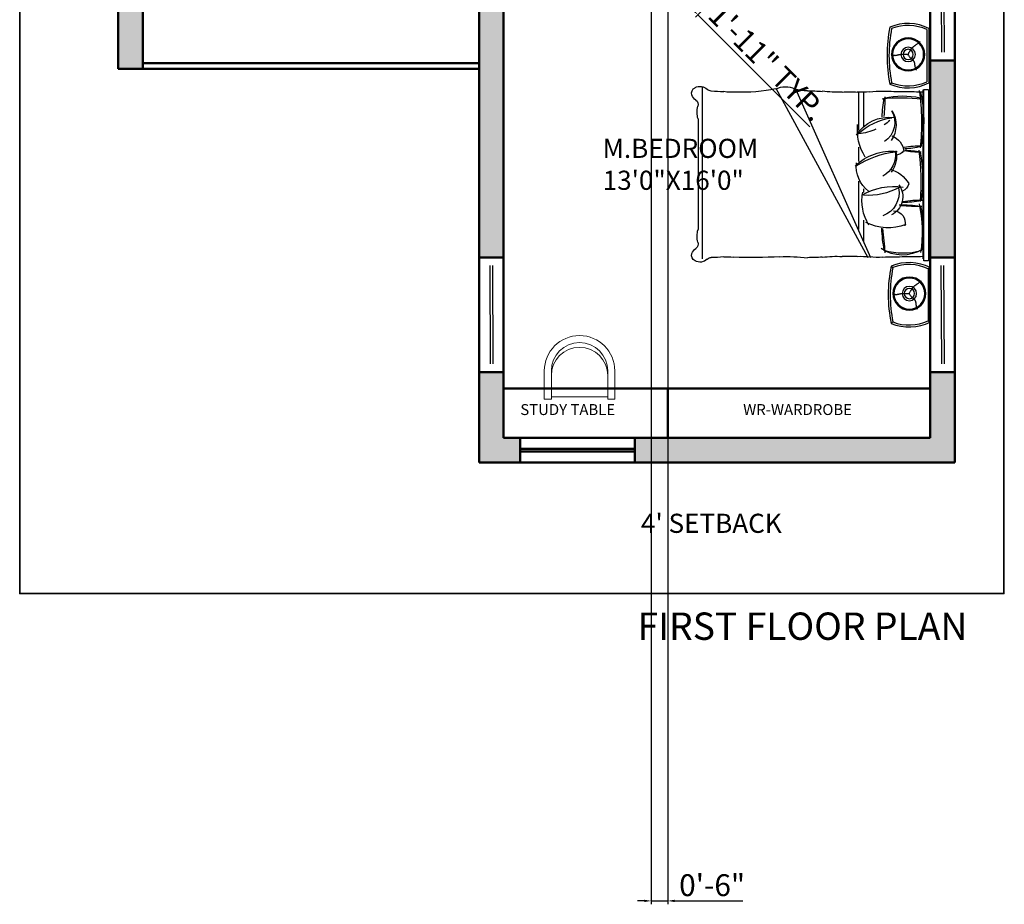
# Model space of a CAD drawing. Units: inches. Extents: x 1986 to 21484, y -1816 to 2016.
# Tile 4 of 85: x 2500 to 2860, y 953 to 1277. Entities that reach past the tile are written whole.
import ezdxf

# ---------------------------------------------------------------- set-up
doc = ezdxf.new("R2010")
doc.units = ezdxf.units.IN
for name, color, linetype, lineweight in [('A-ANNO-DIMS', 2, 'Continuous', 18), ('A-ANNO-TEXT', 7, 'Continuous', 18), ('A-AREA-IDEN', 3, 'Continuous', 18), ('A-FLOR-FIXT', 8, 'Continuous', 18), ('A-FURN', 8, 'Continuous', 18), ('A-GLAZ', 4, 'Continuous', 25), ('A-WALL', 7, 'Continuous', 50), ('A-WALL-PATT', 8, 'Continuous', 13), ('C-PROP', 7, 'Continuous', 35)]:
    doc.layers.add(name, color=color, linetype=linetype, lineweight=lineweight)
doc.layers.add('TEFRİŞ', color=11, linetype='Continuous')
doc.styles.get("Standard").update_dxf_attribs({"font": 'arial.ttf'})
doc.dimstyles.new('ISO-25', dxfattribs={"dimtxt": 8, "dimasz": 2.5, "dimexe": 1.25, "dimexo": 0.625, "dimtad": 1, "dimdec": 1, "dimlunit": 3, "dimtxsty": 'Standard', "dimcen": 2.5, "dimadec": 0, "dimazin": 0, "dimtfac": 1, "dimtdec": 1, "dimtmove": 0, "dimatfit": 3, "dimfxl": 1, "dimarcsym": 0})

# ---------------------------------------------------------------- blocks, each defined once
blk = doc.blocks.new('BED')
at = {"layer": 'TEFRİŞ'}
for p, q in [((2114.88, 1835.66), (2129.12, 1835.66)), ((2115.2, 1835.15), (2128.8, 1835.15)), ((2130.81, 1834.34), (2130.81, 1835.55)), ((2130.91, 1835.55), (2175.56, 1835.55)), ((2175.56, 1835.55), (2175.56, 1834.34)), ((2177.29, 1835.98), (2177.61, 1835.47)), ((2177.29, 1835.98), (2191.52, 1835.98)), ((2177.61, 1835.47), (2191.2, 1835.47)), ((2191.2, 1835.47), (2191.52, 1835.98)), ((2118.49, 1833.2), (2118.34, 1833.38)), ((2118.49, 1833.2), (2118.34, 1833.38)), ((2118.63, 1833.03), (2118.49, 1833.2)), ((2118.63, 1833.03), (2118.49, 1833.2)), ((2118.75, 1832.88), (2118.63, 1833.03)), ((2118.75, 1832.88), (2118.63, 1833.03)), ((2118.86, 1832.74), (2118.75, 1832.88)), ((2118.86, 1832.74), (2118.75, 1832.88)), ((2118.95, 1832.61), (2118.86, 1832.74)), ((2118.95, 1832.61), (2118.86, 1832.74)), ((2119.04, 1832.48), (2118.95, 1832.61)), ((2119.04, 1832.48), (2118.95, 1832.61)), ((2119.12, 1832.37), (2119.04, 1832.48)), ((2119.12, 1832.37), (2119.04, 1832.48)), ((2119.19, 1832.26), (2119.12, 1832.37)), ((2119.19, 1832.26), (2119.12, 1832.37)), ((2119.26, 1832.16), (2119.19, 1832.26)), ((2119.26, 1832.16), (2119.19, 1832.26)), ((2125.52, 1832.21), (2125.6, 1832.25)), ((2125.52, 1832.21), (2125.6, 1832.25)), ((2125.6, 1832.25), (2125.68, 1832.3)), ((2125.6, 1832.25), (2125.68, 1832.3)), ((2125.68, 1832.3), (2125.75, 1832.35)), ((2125.68, 1832.3), (2125.75, 1832.35)), ((2175.56, 1834.34), (2130.81, 1834.34)), ((2175, 1834.19), (2130.91, 1834.19)), ((2180.9, 1833.52), (2180.75, 1833.7)), ((2180.9, 1833.52), (2180.75, 1833.7)), ((2181.04, 1833.35), (2180.9, 1833.52)), ((2181.04, 1833.35), (2180.9, 1833.52)), ((2181.16, 1833.2), (2181.04, 1833.35)), ((2181.16, 1833.2), (2181.04, 1833.35)), ((2181.26, 1833.06), (2181.16, 1833.2)), ((2181.26, 1833.06), (2181.16, 1833.2)), ((2181.36, 1832.93), (2181.26, 1833.06)), ((2181.36, 1832.93), (2181.26, 1833.06)), ((2181.44, 1832.8), (2181.36, 1832.93)), ((2181.44, 1832.8), (2181.36, 1832.93)), ((2181.52, 1832.69), (2181.44, 1832.8)), ((2181.52, 1832.69), (2181.44, 1832.8)), ((2181.59, 1832.58), (2181.52, 1832.69)), ((2181.59, 1832.58), (2181.52, 1832.69)), ((2181.66, 1832.48), (2181.59, 1832.58)), ((2181.66, 1832.48), (2181.59, 1832.58)), ((2181.73, 1832.38), (2181.66, 1832.48)), ((2181.73, 1832.38), (2181.66, 1832.48)), ((2181.79, 1832.29), (2181.73, 1832.38)), ((2181.79, 1832.29), (2181.73, 1832.38)), ((2181.85, 1832.21), (2181.79, 1832.29)), ((2181.85, 1832.21), (2181.79, 1832.29)), ((2186.82, 1832.25), (2186.9, 1832.26)), ((2186.82, 1832.25), (2186.9, 1832.26)), ((2186.9, 1832.26), (2186.97, 1832.27)), ((2186.9, 1832.26), (2186.97, 1832.27)), ((2186.97, 1832.27), (2187.04, 1832.28)), ((2186.97, 1832.27), (2187.04, 1832.28)), ((2187.04, 1832.28), (2187.12, 1832.3)), ((2187.04, 1832.28), (2187.12, 1832.3)), ((2187.12, 1832.3), (2187.2, 1832.31)), ((2187.12, 1832.3), (2187.2, 1832.31)), ((2187.2, 1832.31), (2187.28, 1832.33)), ((2187.2, 1832.31), (2187.28, 1832.33)), ((2187.28, 1832.33), (2187.36, 1832.35)), ((2187.28, 1832.33), (2187.36, 1832.35)), ((2187.36, 1832.35), (2187.45, 1832.37)), ((2187.36, 1832.35), (2187.45, 1832.37)), ((2187.45, 1832.37), (2187.54, 1832.4)), ((2187.45, 1832.37), (2187.54, 1832.4)), ((2187.54, 1832.4), (2187.64, 1832.43)), ((2187.54, 1832.4), (2187.64, 1832.43)), ((2187.64, 1832.43), (2187.74, 1832.46)), ((2187.64, 1832.43), (2187.74, 1832.46)), ((2187.74, 1832.46), (2187.83, 1832.49)), ((2187.74, 1832.46), (2187.83, 1832.49)), ((2187.83, 1832.49), (2187.92, 1832.53)), ((2187.83, 1832.49), (2187.92, 1832.53)), ((2187.92, 1832.53), (2188.01, 1832.57)), ((2187.92, 1832.53), (2188.01, 1832.57)), ((2188.01, 1832.57), (2188.09, 1832.62)), ((2188.01, 1832.57), (2188.09, 1832.62)), ((2188.09, 1832.62), (2188.15, 1832.67)), ((2188.09, 1832.62), (2188.15, 1832.67)), ((2119.32, 1832.06), (2119.26, 1832.16)), ((2119.32, 1832.06), (2119.26, 1832.16)), ((2119.39, 1831.97), (2119.32, 1832.06)), ((2119.39, 1831.97), (2119.32, 1832.06)), ((2119.45, 1831.89), (2119.39, 1831.97)), ((2119.45, 1831.89), (2119.39, 1831.97)), ((2119.51, 1831.81), (2119.45, 1831.89)), ((2119.51, 1831.81), (2119.45, 1831.89)), ((2119.57, 1831.73), (2119.51, 1831.81)), ((2119.57, 1831.73), (2119.51, 1831.81)), ((2119.63, 1831.65), (2119.57, 1831.73)), ((2119.63, 1831.65), (2119.57, 1831.73)), ((2119.69, 1831.58), (2119.63, 1831.65)), ((2119.69, 1831.58), (2119.63, 1831.65)), ((2119.75, 1831.51), (2119.69, 1831.58)), ((2119.75, 1831.51), (2119.69, 1831.58)), ((2119.81, 1831.44), (2119.75, 1831.51)), ((2119.81, 1831.44), (2119.75, 1831.51)), ((2119.87, 1831.38), (2119.81, 1831.44)), ((2119.87, 1831.38), (2119.81, 1831.44)), ((2119.93, 1831.31), (2119.87, 1831.38)), ((2119.93, 1831.31), (2119.87, 1831.38)), ((2119.99, 1831.25), (2119.93, 1831.31)), ((2119.99, 1831.25), (2119.93, 1831.31)), ((2120.05, 1831.2), (2119.99, 1831.25)), ((2120.05, 1831.2), (2119.99, 1831.25)), ((2120.12, 1831.14), (2120.05, 1831.2)), ((2120.12, 1831.14), (2120.05, 1831.2)), ((2120.18, 1831.09), (2120.12, 1831.14)), ((2120.18, 1831.09), (2120.12, 1831.14)), ((2120.25, 1831.04), (2120.18, 1831.09)), ((2120.25, 1831.04), (2120.18, 1831.09)), ((2120.32, 1830.99), (2120.25, 1831.04)), ((2120.32, 1830.99), (2120.25, 1831.04)), ((2120.39, 1830.94), (2120.32, 1830.99)), ((2120.39, 1830.94), (2120.32, 1830.99)), ((2120.47, 1830.9), (2120.39, 1830.94)), ((2120.47, 1830.9), (2120.39, 1830.94)), ((2120.54, 1830.85), (2120.47, 1830.9)), ((2120.54, 1830.85), (2120.47, 1830.9)), ((2120.62, 1830.8), (2120.54, 1830.85)), ((2120.62, 1830.8), (2120.54, 1830.85)), ((2120.7, 1830.75), (2120.62, 1830.8)), ((2120.7, 1830.75), (2120.62, 1830.8)), ((2120.79, 1830.7), (2120.7, 1830.75)), ((2120.79, 1830.7), (2120.7, 1830.75)), ((2120.88, 1830.65), (2120.79, 1830.7)), ((2120.88, 1830.65), (2120.79, 1830.7)), ((2120.98, 1830.59), (2120.88, 1830.65)), ((2120.98, 1830.59), (2120.88, 1830.65)), ((2121.09, 1830.52), (2120.98, 1830.59)), ((2121.09, 1830.52), (2120.98, 1830.59)), ((2121.21, 1830.45), (2121.09, 1830.52)), ((2121.21, 1830.45), (2121.09, 1830.52)), ((2121.34, 1830.38), (2121.21, 1830.45)), ((2121.34, 1830.38), (2121.21, 1830.45)), ((2121.49, 1830.29), (2121.34, 1830.38)), ((2121.49, 1830.29), (2121.34, 1830.38)), ((2121.66, 1830.21), (2121.49, 1830.29)), ((2121.66, 1830.21), (2121.49, 1830.29)), ((2121.66, 1830.18), (2121.87, 1830.29)), ((2121.66, 1830.18), (2121.87, 1830.29)), ((2121.85, 1830.11), (2121.66, 1830.21)), ((2121.85, 1830.11), (2121.66, 1830.21)), ((2121.74, 1829.99), (2121.73, 1829.83)), ((2121.74, 1829.99), (2121.73, 1829.83)), ((2121.73, 1829.83), (2121.73, 1829.69)), ((2121.73, 1829.83), (2121.73, 1829.69)), ((2121.73, 1829.69), (2121.73, 1829.57)), ((2121.73, 1829.69), (2121.73, 1829.57)), ((2121.76, 1830.38), (2121.74, 1830.17)), ((2121.76, 1830.38), (2121.74, 1830.17)), ((2121.74, 1830.17), (2121.74, 1829.99)), ((2121.74, 1830.17), (2121.74, 1829.99)), ((2121.87, 1830.29), (2122.04, 1830.4)), ((2121.87, 1830.29), (2122.04, 1830.4)), ((2122.04, 1830.4), (2122.2, 1830.51)), ((2122.04, 1830.4), (2122.2, 1830.51)), ((2122.2, 1830.51), (2122.33, 1830.61)), ((2122.2, 1830.51), (2122.33, 1830.61)), ((2122.33, 1830.61), (2122.45, 1830.72)), ((2122.33, 1830.61), (2122.45, 1830.72)), ((2122.45, 1830.72), (2122.55, 1830.82)), ((2122.45, 1830.72), (2122.55, 1830.82)), ((2122.55, 1830.82), (2122.64, 1830.91)), ((2122.55, 1830.82), (2122.64, 1830.91)), ((2122.64, 1830.91), (2122.72, 1831.01)), ((2122.64, 1830.91), (2122.72, 1831.01)), ((2122.72, 1831.01), (2122.8, 1831.09)), ((2122.72, 1831.01), (2122.8, 1831.09)), ((2122.8, 1831.09), (2122.87, 1831.18)), ((2122.8, 1831.09), (2122.87, 1831.18)), ((2122.87, 1831.18), (2122.94, 1831.26)), ((2122.87, 1831.18), (2122.94, 1831.26)), ((2122.94, 1831.26), (2123.01, 1831.33)), ((2122.94, 1831.26), (2123.01, 1831.33)), ((2123.01, 1831.33), (2123.08, 1831.4)), ((2123.01, 1831.33), (2123.08, 1831.4)), ((2123.08, 1831.4), (2123.14, 1831.46)), ((2123.08, 1831.4), (2123.14, 1831.46)), ((2123.14, 1831.46), (2123.21, 1831.52)), ((2123.14, 1831.46), (2123.21, 1831.52)), ((2123.21, 1831.52), (2123.27, 1831.58)), ((2123.21, 1831.52), (2123.27, 1831.58)), ((2123.27, 1831.58), (2123.34, 1831.63)), ((2123.27, 1831.58), (2123.34, 1831.63)), ((2123.34, 1831.63), (2123.41, 1831.67)), ((2123.34, 1831.63), (2123.41, 1831.67)), ((2123.41, 1831.67), (2123.48, 1831.71)), ((2123.41, 1831.67), (2123.48, 1831.71)), ((2123.48, 1831.71), (2123.55, 1831.74)), ((2123.48, 1831.71), (2123.55, 1831.74)), ((2123.55, 1831.74), (2123.62, 1831.77)), ((2123.55, 1831.74), (2123.62, 1831.77)), ((2123.62, 1831.77), (2123.69, 1831.8)), ((2123.62, 1831.77), (2123.69, 1831.8)), ((2123.69, 1831.8), (2123.77, 1831.82)), ((2123.69, 1831.8), (2123.77, 1831.82)), ((2123.77, 1831.82), (2123.84, 1831.84)), ((2123.77, 1831.82), (2123.84, 1831.84)), ((2123.84, 1831.84), (2123.91, 1831.86)), ((2123.84, 1831.84), (2123.91, 1831.86)), ((2123.91, 1831.86), (2123.98, 1831.87)), ((2123.91, 1831.86), (2123.98, 1831.87)), ((2123.98, 1831.87), (2124.06, 1831.89)), ((2123.98, 1831.87), (2124.06, 1831.89)), ((2124.06, 1831.89), (2124.13, 1831.9)), ((2124.06, 1831.89), (2124.13, 1831.9)), ((2124.13, 1831.9), (2124.2, 1831.91)), ((2124.13, 1831.9), (2124.2, 1831.91)), ((2124.2, 1831.91), (2124.27, 1831.91)), ((2124.2, 1831.91), (2124.27, 1831.91)), ((2124.27, 1831.91), (2124.35, 1831.92)), ((2124.27, 1831.91), (2124.35, 1831.92)), ((2124.35, 1831.92), (2124.42, 1831.93)), ((2124.35, 1831.92), (2124.42, 1831.93)), ((2124.42, 1831.93), (2124.49, 1831.94)), ((2124.42, 1831.93), (2124.49, 1831.94)), ((2124.49, 1831.94), (2124.56, 1831.95)), ((2124.49, 1831.94), (2124.56, 1831.95)), ((2124.56, 1831.95), (2124.64, 1831.96)), ((2124.56, 1831.95), (2124.64, 1831.96)), ((2124.64, 1831.96), (2124.71, 1831.98)), ((2124.64, 1831.96), (2124.71, 1831.98)), ((2124.71, 1831.98), (2124.79, 1831.99)), ((2124.71, 1831.98), (2124.79, 1831.99)), ((2124.79, 1831.99), (2124.87, 1832.01)), ((2124.79, 1831.99), (2124.87, 1832.01)), ((2124.87, 1832.01), (2124.96, 1832.03)), ((2124.87, 1832.01), (2124.96, 1832.03)), ((2124.96, 1832.03), (2125.05, 1832.05)), ((2124.96, 1832.03), (2125.05, 1832.05)), ((2125.05, 1832.05), (2125.14, 1832.08)), ((2125.05, 1832.05), (2125.14, 1832.08)), ((2125.14, 1832.08), (2125.23, 1832.11)), ((2125.14, 1832.08), (2125.23, 1832.11)), ((2125.23, 1832.11), (2125.33, 1832.14)), ((2125.23, 1832.11), (2125.33, 1832.14)), ((2125.33, 1832.14), (2125.42, 1832.17)), ((2125.33, 1832.14), (2125.42, 1832.17)), ((2125.42, 1832.17), (2125.52, 1832.21)), ((2125.42, 1832.17), (2125.52, 1832.21)), ((2181.92, 1832.13), (2181.85, 1832.21)), ((2181.92, 1832.13), (2181.85, 1832.21)), ((2181.97, 1832.05), (2181.92, 1832.13)), ((2181.97, 1832.05), (2181.92, 1832.13)), ((2182.03, 1831.97), (2181.97, 1832.05)), ((2182.03, 1831.97), (2181.97, 1832.05)), ((2182.09, 1831.9), (2182.03, 1831.97)), ((2182.09, 1831.9), (2182.03, 1831.97)), ((2182.15, 1831.83), (2182.09, 1831.9)), ((2182.15, 1831.83), (2182.09, 1831.9)), ((2182.21, 1831.76), (2182.15, 1831.83)), ((2182.21, 1831.76), (2182.15, 1831.83)), ((2182.27, 1831.7), (2182.21, 1831.76)), ((2182.27, 1831.7), (2182.21, 1831.76)), ((2182.33, 1831.63), (2182.27, 1831.7)), ((2182.33, 1831.63), (2182.27, 1831.7)), ((2182.4, 1831.57), (2182.33, 1831.63)), ((2182.4, 1831.57), (2182.33, 1831.63)), ((2182.46, 1831.52), (2182.4, 1831.57)), ((2182.46, 1831.52), (2182.4, 1831.57)), ((2182.52, 1831.46), (2182.46, 1831.52)), ((2182.52, 1831.46), (2182.46, 1831.52)), ((2182.59, 1831.41), (2182.52, 1831.46)), ((2182.59, 1831.41), (2182.52, 1831.46)), ((2182.66, 1831.36), (2182.59, 1831.41)), ((2182.66, 1831.36), (2182.59, 1831.41)), ((2182.73, 1831.31), (2182.66, 1831.36)), ((2182.73, 1831.31), (2182.66, 1831.36)), ((2182.8, 1831.26), (2182.73, 1831.31)), ((2182.8, 1831.26), (2182.73, 1831.31)), ((2182.87, 1831.22), (2182.8, 1831.26)), ((2182.87, 1831.22), (2182.8, 1831.26)), ((2182.95, 1831.17), (2182.87, 1831.22)), ((2182.95, 1831.17), (2182.87, 1831.22)), ((2183.03, 1831.12), (2182.95, 1831.17)), ((2183.03, 1831.12), (2182.95, 1831.17)), ((2183.11, 1831.07), (2183.03, 1831.12)), ((2183.11, 1831.07), (2183.03, 1831.12)), ((2183.2, 1831.02), (2183.11, 1831.07)), ((2183.2, 1831.02), (2183.11, 1831.07)), ((2183.29, 1830.97), (2183.2, 1831.02)), ((2183.29, 1830.97), (2183.2, 1831.02)), ((2183.39, 1830.91), (2183.29, 1830.97)), ((2183.39, 1830.91), (2183.29, 1830.97)), ((2183.49, 1830.84), (2183.39, 1830.91)), ((2183.49, 1830.84), (2183.39, 1830.91)), ((2183.61, 1830.77), (2183.49, 1830.84)), ((2183.61, 1830.77), (2183.49, 1830.84)), ((2183.75, 1830.7), (2183.61, 1830.77)), ((2183.75, 1830.7), (2183.61, 1830.77)), ((2183.9, 1830.61), (2183.75, 1830.7)), ((2183.9, 1830.61), (2183.75, 1830.7)), ((2184.06, 1830.53), (2183.9, 1830.61)), ((2184.06, 1830.53), (2183.9, 1830.61)), ((2184.25, 1830.43), (2184.06, 1830.53)), ((2184.25, 1830.43), (2184.06, 1830.53)), ((2184.07, 1830.5), (2184.27, 1830.61)), ((2184.07, 1830.5), (2184.27, 1830.61)), ((2184.15, 1830.49), (2184.14, 1830.31)), ((2184.15, 1830.49), (2184.14, 1830.31)), ((2184.14, 1830.31), (2184.14, 1830.15)), ((2184.14, 1830.31), (2184.14, 1830.15)), ((2184.14, 1830.15), (2184.14, 1830.01)), ((2184.14, 1830.15), (2184.14, 1830.01)), ((2184.14, 1830.01), (2184.14, 1829.89)), ((2184.14, 1830.01), (2184.14, 1829.89)), ((2184.14, 1829.89), (2184.14, 1829.77)), ((2184.14, 1829.89), (2184.14, 1829.77)), ((2184.14, 1829.77), (2184.14, 1829.67)), ((2184.14, 1829.77), (2184.14, 1829.67)), ((2184.17, 1830.7), (2184.15, 1830.49)), ((2184.17, 1830.7), (2184.15, 1830.49)), ((2184.27, 1830.61), (2184.45, 1830.72)), ((2184.27, 1830.61), (2184.45, 1830.72)), ((2184.45, 1830.72), (2184.6, 1830.83)), ((2184.45, 1830.72), (2184.6, 1830.83)), ((2184.6, 1830.83), (2184.74, 1830.93)), ((2184.6, 1830.83), (2184.74, 1830.93)), ((2184.74, 1830.93), (2184.85, 1831.04)), ((2184.74, 1830.93), (2184.85, 1831.04)), ((2184.85, 1831.04), (2184.95, 1831.14)), ((2184.85, 1831.04), (2184.95, 1831.14)), ((2184.95, 1831.14), (2185.05, 1831.23)), ((2184.95, 1831.14), (2185.05, 1831.23)), ((2185.05, 1831.23), (2185.13, 1831.33)), ((2185.05, 1831.23), (2185.13, 1831.33)), ((2185.13, 1831.33), (2185.21, 1831.41)), ((2185.13, 1831.33), (2185.21, 1831.41)), ((2185.21, 1831.41), (2185.28, 1831.5)), ((2185.21, 1831.41), (2185.28, 1831.5)), ((2185.28, 1831.5), (2185.35, 1831.58)), ((2185.28, 1831.5), (2185.35, 1831.58)), ((2185.35, 1831.58), (2185.42, 1831.65)), ((2185.35, 1831.58), (2185.42, 1831.65)), ((2185.42, 1831.65), (2185.48, 1831.72)), ((2185.42, 1831.65), (2185.48, 1831.72)), ((2185.48, 1831.72), (2185.55, 1831.78)), ((2185.48, 1831.72), (2185.55, 1831.78)), ((2185.55, 1831.78), (2185.61, 1831.84)), ((2185.55, 1831.78), (2185.61, 1831.84)), ((2185.61, 1831.84), (2185.68, 1831.9)), ((2185.61, 1831.84), (2185.68, 1831.9)), ((2185.68, 1831.9), (2185.75, 1831.95)), ((2185.68, 1831.9), (2185.75, 1831.95)), ((2185.75, 1831.95), (2185.82, 1831.99)), ((2185.75, 1831.95), (2185.82, 1831.99)), ((2185.82, 1831.99), (2185.89, 1832.03)), ((2185.82, 1831.99), (2185.89, 1832.03)), ((2185.89, 1832.03), (2185.96, 1832.06)), ((2185.89, 1832.03), (2185.96, 1832.06)), ((2185.96, 1832.06), (2186.03, 1832.09)), ((2185.96, 1832.06), (2186.03, 1832.09)), ((2186.03, 1832.09), (2186.1, 1832.12)), ((2186.03, 1832.09), (2186.1, 1832.12)), ((2186.1, 1832.12), (2186.17, 1832.14)), ((2186.1, 1832.12), (2186.17, 1832.14)), ((2186.17, 1832.14), (2186.24, 1832.16)), ((2186.17, 1832.14), (2186.24, 1832.16)), ((2186.24, 1832.16), (2186.32, 1832.18)), ((2186.24, 1832.16), (2186.32, 1832.18)), ((2186.32, 1832.18), (2186.39, 1832.19)), ((2186.32, 1832.18), (2186.39, 1832.19)), ((2186.39, 1832.19), (2186.46, 1832.21)), ((2186.39, 1832.19), (2186.46, 1832.21)), ((2186.46, 1832.21), (2186.53, 1832.22)), ((2186.46, 1832.21), (2186.53, 1832.22)), ((2186.53, 1832.22), (2186.61, 1832.23)), ((2186.53, 1832.22), (2186.61, 1832.23)), ((2186.61, 1832.23), (2186.68, 1832.23)), ((2186.61, 1832.23), (2186.68, 1832.23)), ((2186.68, 1832.23), (2186.75, 1832.24)), ((2186.68, 1832.23), (2186.75, 1832.24)), ((2186.75, 1832.24), (2186.82, 1832.25)), ((2186.75, 1832.24), (2186.82, 1832.25)), ((2121.73, 1829.57), (2121.73, 1829.45)), ((2121.73, 1829.57), (2121.73, 1829.45)), ((2121.73, 1829.45), (2121.74, 1829.35)), ((2121.73, 1829.45), (2121.74, 1829.35)), ((2121.74, 1828.89), (2121.73, 1828.8)), ((2121.74, 1828.89), (2121.73, 1828.8)), ((2121.73, 1828.8), (2121.73, 1828.72)), ((2121.73, 1828.8), (2121.73, 1828.72)), ((2121.73, 1828.72), (2121.73, 1828.64)), ((2121.73, 1828.72), (2121.73, 1828.64)), ((2121.73, 1828.64), (2121.73, 1828.56)), ((2121.73, 1828.64), (2121.73, 1828.56)), ((2121.73, 1828.56), (2121.73, 1828.48)), ((2121.73, 1828.56), (2121.73, 1828.48)), ((2121.73, 1828.48), (2121.73, 1828.4)), ((2121.73, 1828.48), (2121.73, 1828.4)), ((2121.73, 1828.4), (2121.73, 1828.33)), ((2121.73, 1828.4), (2121.73, 1828.33)), ((2121.73, 1828.33), (2121.74, 1828.25)), ((2121.73, 1828.33), (2121.74, 1828.25)), ((2121.74, 1829.35), (2121.74, 1829.25)), ((2121.74, 1829.35), (2121.74, 1829.25)), ((2121.74, 1829.25), (2121.74, 1829.16)), ((2121.74, 1829.25), (2121.74, 1829.16)), ((2121.74, 1829.16), (2121.74, 1829.06)), ((2121.74, 1829.16), (2121.74, 1829.06)), ((2121.74, 1829.06), (2121.74, 1828.97)), ((2121.74, 1829.06), (2121.74, 1828.97)), ((2121.74, 1828.97), (2121.74, 1828.89)), ((2121.74, 1828.97), (2121.74, 1828.89)), ((2121.74, 1828.25), (2121.75, 1828.18)), ((2121.74, 1828.25), (2121.75, 1828.18)), ((2121.75, 1828.18), (2121.75, 1828.1)), ((2121.75, 1828.18), (2121.75, 1828.1)), ((2121.75, 1828.1), (2121.76, 1828.03)), ((2121.75, 1828.1), (2121.76, 1828.03)), ((2121.76, 1828.03), (2121.78, 1827.95)), ((2121.76, 1828.03), (2121.78, 1827.95)), ((2121.78, 1827.95), (2121.79, 1827.88)), ((2121.78, 1827.95), (2121.79, 1827.88)), ((2121.79, 1827.88), (2121.8, 1827.8)), ((2121.79, 1827.88), (2121.8, 1827.8)), ((2121.8, 1827.8), (2121.82, 1827.72)), ((2121.8, 1827.8), (2121.82, 1827.72)), ((2121.82, 1827.72), (2121.84, 1827.65)), ((2121.82, 1827.72), (2121.84, 1827.65)), ((2121.84, 1827.65), (2121.85, 1827.57)), ((2121.84, 1827.65), (2121.85, 1827.57)), ((2121.85, 1827.57), (2121.87, 1827.49)), ((2121.85, 1827.57), (2121.87, 1827.49)), ((2121.87, 1827.49), (2121.89, 1827.41)), ((2121.87, 1827.49), (2121.89, 1827.41)), ((2121.89, 1827.41), (2121.91, 1827.33)), ((2121.89, 1827.41), (2121.91, 1827.33)), ((2121.91, 1827.33), (2121.93, 1827.26)), ((2121.91, 1827.33), (2121.93, 1827.26)), ((2121.93, 1827.26), (2121.95, 1827.18)), ((2121.93, 1827.26), (2121.95, 1827.18)), ((2121.95, 1827.18), (2121.97, 1827.09)), ((2121.95, 1827.18), (2121.97, 1827.09)), ((2184.14, 1829.04), (2184.13, 1828.96)), ((2184.14, 1829.04), (2184.13, 1828.96)), ((2184.13, 1828.96), (2184.13, 1828.88)), ((2184.13, 1828.96), (2184.13, 1828.88)), ((2184.13, 1828.88), (2184.13, 1828.8)), ((2184.13, 1828.88), (2184.13, 1828.8)), ((2184.13, 1828.8), (2184.14, 1828.72)), ((2184.13, 1828.8), (2184.14, 1828.72)), ((2184.14, 1829.67), (2184.15, 1829.57)), ((2184.14, 1829.67), (2184.15, 1829.57)), ((2184.15, 1829.38), (2184.14, 1829.29)), ((2184.15, 1829.38), (2184.14, 1829.29)), ((2184.14, 1829.29), (2184.14, 1829.21)), ((2184.14, 1829.29), (2184.14, 1829.21)), ((2184.14, 1829.21), (2184.14, 1829.12)), ((2184.14, 1829.21), (2184.14, 1829.12)), ((2184.14, 1829.12), (2184.14, 1829.04)), ((2184.14, 1829.12), (2184.14, 1829.04)), ((2184.14, 1828.72), (2184.14, 1828.65)), ((2184.14, 1828.72), (2184.14, 1828.65)), ((2184.14, 1828.65), (2184.15, 1828.57)), ((2184.14, 1828.65), (2184.15, 1828.57)), ((2184.15, 1829.57), (2184.15, 1829.48)), ((2184.15, 1829.57), (2184.15, 1829.48)), ((2184.15, 1829.48), (2184.15, 1829.38)), ((2184.15, 1829.48), (2184.15, 1829.38)), ((2184.15, 1828.57), (2184.15, 1828.5)), ((2184.15, 1828.57), (2184.15, 1828.5)), ((2184.15, 1828.5), (2184.16, 1828.42)), ((2184.15, 1828.5), (2184.16, 1828.42)), ((2184.16, 1828.42), (2184.17, 1828.35)), ((2184.16, 1828.42), (2184.17, 1828.35)), ((2184.17, 1828.35), (2184.18, 1828.27)), ((2184.17, 1828.35), (2184.18, 1828.27)), ((2184.18, 1828.27), (2184.19, 1828.2)), ((2184.18, 1828.27), (2184.19, 1828.2)), ((2184.19, 1828.2), (2184.21, 1828.12)), ((2184.19, 1828.2), (2184.21, 1828.12)), ((2184.21, 1828.12), (2184.22, 1828.04)), ((2184.21, 1828.12), (2184.22, 1828.04)), ((2184.22, 1828.04), (2184.24, 1827.97)), ((2184.22, 1828.04), (2184.24, 1827.97)), ((2184.24, 1827.97), (2184.26, 1827.89)), ((2184.24, 1827.97), (2184.26, 1827.89)), ((2184.26, 1827.89), (2184.28, 1827.81)), ((2184.26, 1827.89), (2184.28, 1827.81)), ((2184.28, 1827.81), (2184.3, 1827.73)), ((2184.28, 1827.81), (2184.3, 1827.73)), ((2184.3, 1827.73), (2184.32, 1827.65)), ((2184.3, 1827.73), (2184.32, 1827.65)), ((2184.32, 1827.65), (2184.34, 1827.58)), ((2184.32, 1827.65), (2184.34, 1827.58)), ((2184.34, 1827.58), (2184.36, 1827.5)), ((2184.34, 1827.58), (2184.36, 1827.5)), ((2184.36, 1827.5), (2184.38, 1827.41)), ((2184.36, 1827.5), (2184.38, 1827.41)), ((2184.38, 1827.41), (2184.4, 1827.33)), ((2184.38, 1827.41), (2184.4, 1827.33)), ((2184.4, 1827.33), (2184.41, 1827.25)), ((2184.4, 1827.33), (2184.41, 1827.25)), ((2184.41, 1827.25), (2184.41, 1827.16)), ((2184.41, 1827.25), (2184.41, 1827.16)), ((2184.41, 1827.16), (2184.41, 1827.06)), ((2184.41, 1827.16), (2184.41, 1827.06)), ((2121.78, 1825.93), (2121.74, 1825.8)), ((2121.78, 1825.93), (2121.74, 1825.8)), ((2121.83, 1826.06), (2121.78, 1825.93)), ((2121.83, 1826.06), (2121.78, 1825.93)), ((2121.87, 1826.19), (2121.83, 1826.06)), ((2121.87, 1826.19), (2121.83, 1826.06)), ((2121.91, 1826.31), (2121.87, 1826.19)), ((2121.91, 1826.31), (2121.87, 1826.19)), ((2121.95, 1826.42), (2121.91, 1826.31)), ((2121.95, 1826.42), (2121.91, 1826.31)), ((2121.97, 1826.54), (2121.95, 1826.42)), ((2121.97, 1826.54), (2121.95, 1826.42)), ((2121.97, 1827.09), (2121.99, 1827.01)), ((2121.97, 1827.09), (2121.99, 1827.01)), ((2121.99, 1826.64), (2121.97, 1826.54)), ((2121.99, 1826.64), (2121.97, 1826.54)), ((2121.99, 1827.01), (2122, 1826.93)), ((2121.99, 1827.01), (2122, 1826.93)), ((2122, 1826.74), (2121.99, 1826.64)), ((2122, 1826.74), (2121.99, 1826.64)), ((2122, 1826.93), (2122.01, 1826.84)), ((2122, 1826.93), (2122.01, 1826.84)), ((2122.01, 1826.84), (2122, 1826.74)), ((2122.01, 1826.84), (2122, 1826.74)), ((2129.46, 1825.49), (2129.09, 1825.93)), ((2176.94, 1825.81), (2177.31, 1826.25)), ((2184.19, 1826.25), (2184.14, 1826.12)), ((2184.19, 1826.25), (2184.14, 1826.12)), ((2184.23, 1826.38), (2184.19, 1826.25)), ((2184.23, 1826.38), (2184.19, 1826.25)), ((2184.28, 1826.51), (2184.23, 1826.38)), ((2184.28, 1826.51), (2184.23, 1826.38)), ((2184.32, 1826.63), (2184.28, 1826.51)), ((2184.32, 1826.63), (2184.28, 1826.51)), ((2184.35, 1826.74), (2184.32, 1826.63)), ((2184.35, 1826.74), (2184.32, 1826.63)), ((2184.38, 1826.86), (2184.35, 1826.74)), ((2184.38, 1826.86), (2184.35, 1826.74)), ((2184.4, 1826.96), (2184.38, 1826.86)), ((2184.4, 1826.96), (2184.38, 1826.86)), ((2184.41, 1827.06), (2184.4, 1826.96)), ((2184.41, 1827.06), (2184.4, 1826.96)), ((2191.87, 1825.81), (2191.5, 1826.25)), ((2174.77, 1819.77), (2130.6, 1795.83)), ((2174.77, 1820.53), (2130.76, 1800.91)), ((2140.43, 1818.69), (2131.53, 1818.69)), ((2141.43, 1817.4), (2131.53, 1817.4)), ((2149.62, 1817.4), (2145.88, 1817.4)), ((2167.36, 1817.4), (2154.77, 1817.4)), ((2157.71, 1818.69), (2156.77, 1818.69)), ((2170.41, 1818.69), (2164.92, 1818.69)), ((2175, 1776.57), (2130.11, 1776.57)), ((2138.52, 1775.41), (2167.39, 1775.41))]:
    blk.add_line(p, q, dxfattribs=at)
for centre, radius, start, end in [((2126, 1830.19), 12.39, 153.8162, 202.314), ((2126, 1830.19), 11.88, 155.3335, 201.0157), ((2118, 1830.19), 11.88, 338.9843, 24.6665), ((2118, 1830.19), 12.39, 337.686, 26.1838), ((2188.4, 1830.51), 12.39, 153.8162, 202.314), ((2188.4, 1830.51), 11.88, 155.3335, 201.0157), ((2180.41, 1830.51), 11.88, 338.9843, 24.6665), ((2180.41, 1830.51), 12.39, 337.686, 26.1838), ((2122, 1861.35), 36.63, 258.2443, 281.7557), ((2122, 1861.35), 36.12, 258.6773, 281.3227), ((2184.41, 1861.67), 36.63, 258.2443, 281.7557), ((2184.41, 1861.67), 36.12, 258.6773, 281.3227)]:
    blk.add_arc(centre, radius, start, end, dxfattribs=at)
at = {"layer": 'TEFRİŞ', "extrusion": (0, 0, -1)}
for centre, major_axis, ratio, start_param, end_param in [((2184.09, 1830.56), (-3.05, -3.05), 1, 3.926991, 10.210176), ((2184.09, 1830.56), (2.86, -2.86), 1, 5.497787, 11.780972), ((2184.09, 1830.56), (2.86, -2.86), 1, 5.497787, 11.780972), ((2121.68, 1830.24), (-3.05, -3.05), 1, 3.926991, 10.210176), ((2121.68, 1830.24), (2.86, -2.86), 1, 5.497787, 11.780972), ((2121.68, 1830.24), (2.86, -2.86), 1, 5.497787, 11.780972), ((2139.43, 1773.84), (-42.35, 42.35), 1, 0.646251, 0.896949), ((2206.14, 1830.73), (-52.86, -52.86), 1, 0.767743, 0.83177), ((2138.85, 1803.05), (-22.1, 22.1), 1, 0.544604, 1.006234), ((2154.7, 1828.89), (-15.68, 15.68), 1, -1.00675, -0.580436), ((2181.61, 1828.44), (-34.39, 34.39), 1, -0.888486, -0.672463), ((2164.51, 1832.79), (-13.41, 13.41), 1, -0.974476, -0.730892), ((2127.6, 1828.81), (-13.23, 13.23), 1, 2.100388, 2.328052), ((2155, 1761.9), (-50.65, -50.65), 1, 2.239512, 2.426533), ((2172.01, 1828.66), (-17.93, 17.93), 1, -0.753394, -0.598744), ((2128.44, 1832.96), (-13.26, -13.26), 1, 3.889049, 4.127298), ((2154.12, 1796.61), (-26.46, 26.46), 1, 0.596409, 0.940188), ((2183.72, 1833.22), (-17, 17), 1, -0.967105, -0.749712), ((2134, 1828.8), (-18.62, 18.62), 1, 2.173461, 2.355043), ((2168.35, 1789.27), (-1.33, 44.62), 0.875277, -0.163954, 0.163954), ((2199.2, 1828.45), (-27.06, -27.06), 1, 0.770625, 0.917228), ((2087.32, 1833.96), (-52.37, 52.37), 1, 2.358049, 2.431787), ((2167.6, 1797.72), (-0.51, 36.47), 0.865194, -0.185965, 0.185965), ((2164.15, 1828.7), (-6.99, 6.99), 1, 1.789136, 2.946702), ((2156.76, 1828.98), (-11.9, -11.9), 1, 3.646453, 4.226155), ((2099.77, 1830.73), (-52.86, 52.86), 1, 2.311571, 2.373849), ((2184.09, 1830.56), (1.33, -1.33), 1, 5.497787, 11.780972), ((2184.09, 1830.56), (1.33, -1.33), 1, 5.497787, 11.780972), ((2121.68, 1830.24), (1.33, -1.33), 1, 5.497787, 11.780972), ((2121.68, 1830.24), (1.33, -1.33), 1, 5.497787, 11.780972), ((2121.68, 1830.24), (0.952, -0.952), 1, 5.497787, 11.780972), ((2121.68, 1830.24), (0.952, -0.952), 1, 5.497787, 11.780972), ((2159.55, 1823.33), (-5.81, 5.81), 1, -0.516587, 0.256776), ((2154.84, 1827.75), (-1.93, 1.93), 1, 0.997904, 1.977819), ((2166.67, 1824.96), (-2.93, 3.91), 0.760601, -0.723751, 0.723751), ((2184.09, 1830.56), (0.952, -0.952), 1, 5.497787, 11.780972), ((2184.09, 1830.56), (0.952, -0.952), 1, 5.497787, 11.780972), ((2675.38, 1815.09), (-384.79, -384.79), 1, 0.80103, 0.811711), ((2140.05, 1819.86), (-5.1, 5.1), 1, 0.238357, 1.390139), ((2139.42, 1820.79), (-4.21, -4.21), 1, 1.82161, 3.349145), ((2147.44, 1824.41), (-3.36, -3.36), 1, 1.11934, 2.270556), ((2160.6, 1825.98), (-9.68, -9.68), 1, 0.009196, 0.886853), ((2145.66, 1827.01), (-1.62, 1.62), 1, 1.310976, 2.284591), ((2148.35, 1820.65), (-4.63, -4.63), 1, 2.117602, 3.020837), ((2147.86, 1820.64), (-4.48, 4.48), 1, 0.665914, 1.867503), ((2172, 1826.44), (-11.23, 11.23), 1, -1.332486, -0.624868), ((2158.82, 1823.55), (-3.74, -3.74), 1, 1.730792, 3.47045), ((2141.71, 1819.83), (-11.86, 11.86), 1, 1.850844, 2.42862), ((2157.83, 1821.53), (-4.47, 4.47), 1, 0.576679, 2.021689), ((2153.88, 1825.05), (-9.22, 9.22), 1, 1.994956, 2.818753), ((1630.53, 1815.09), (-384.79, 384.79), 1, 2.329881, 2.340562), ((2148.15, 1825.25), (-7.14, -7.14), 1, 6.061986, 7.190757), ((2154.93, 1828.48), (-11.96, 11.96), 1, -1.530302, -0.934407), ((2127.37, 1815.76), (-10.68, 10.68), 1, 1.657204, 1.779381), ((2170.68, 1829.67), (-16.79, 16.79), 1, -1.354718, -0.902276), ((2146.08, 1822.57), (-10.5, 10.5), 1, -0.951783, -0.716225), ((2132.43, 1774.09), (-35.41, -35.41), 1, 2.362911, 2.464592), ((2140.17, 1862.96), (-27.99, 27.99), 1, 3.983025, 4.107469), ((2165.73, 1860.69), (-26.41, -26.41), 1, 5.306413, 5.463767), ((2199.62, 1529.47), (-209.2, 209.2), 1, 0.675361, 0.697001), ((2159.82, 1822.57), (-10.5, -10.5), 1, 3.857817, 4.093375), ((2111.06, 1818.12), (-14.48, 14.48), 1, 2.258605, 2.412359), ((2127.37, 1815.76), (-10.68, 10.68), 1, 1.94252, 2.248924), ((2150.79, 1825.18), (-6, 6), 1, 3.032122, 4.026148), ((2159.02, 1834.9), (-3.04, 16.53), 0.830169, 2.822117, 3.461068), ((2194.85, 1818.12), (-14.48, 14.48), 1, -0.841563, -0.687809), ((2169.92, 1815.01), (-27.2, -27.2), 1, 0.734393, 0.836404), ((2141.33, 1830.48), (-9.55, -9.55), 1, 4.941413, 5.601673), ((2135.98, 1815.01), (-27.2, -27.2), 1, 3.875985, 3.977996), ((2098.24, 1811.68), (-23.54, -23.54), 1, 3.885834, 4.043401), ((2207.66, 1811.68), (-23.54, -23.54), 1, 0.668988, 0.826555), ((2189.03, 1803.74), (-40.91, -40.91), 1, 0.789771, 0.855756), ((2116.87, 1803.74), (-40.91, 40.91), 1, 2.285836, 2.351822), ((2122.14, 1803.63), (-6.39, -6.39), 1, 3.886359, 4.265474), ((2222.76, 1798.77), (-34.16, -34.16), 1, 0.743488, 0.893627), ((2135.02, 1798.41), (-3.45, 3.45), 1, -0.831635, -0.314979), ((2135.48, 1798), (-3.77, -3.77), 1, 0.329385, 0.820948), ((2148.06, 1790.38), (-0.75, 67.37), 0.394952, 1.480524, 1.661068), ((2127.76, 1790.23), (-1, 12.37), 0.296708, 1.141067, 2.000525), ((2118.49, 1784.2), (-9.24, -9.24), 1, 3.839645, 4.088086), ((2182.27, 1782.99), (-5.52, -5.52), 1, 0.671703, 0.993321), ((2162.12, 1778.86), (-21.85, 21.85), 1, -0.78611, -0.680117), ((2143.78, 1778.86), (-21.85, 21.85), 1, 2.250913, 2.356906), ((2129.83, 1778.8), (-0.986, 0.986), 1, 2.330985, 3.163296), ((2176.08, 1778.8), (-0.986, 0.986), 1, 4.690686, 5.522997), ((2132.72, 1775.92), (-1.91, -1.91), 1, 0.284117, 1.557111), ((2173.18, 1775.92), (-1.91, -1.91), 1, 3.155278, 4.428271), ((2131.79, 1775.28), (-1.11, 1.11), 1, 3.629269, 5.067473), ((2130.83, 1777), (-2.49, -2.49), 1, 4.590984, 5.084038), ((2134.73, 1774.06), (-0.964, -0.964), 1, 1.381176, 2.701227), ((2136.75, 1781.14), (-4.24, 4.24), 1, 3.62713, 4.188813), ((2169.16, 1781.14), (-4.24, 4.24), 1, 3.665169, 4.226852), ((2171.17, 1774.06), (-0.964, -0.964), 1, 2.011162, 3.331212), ((2175.07, 1777), (-2.49, 2.49), 1, 4.34074, 4.833793), ((2174.12, 1775.28), (-1.11, 1.11), 1, 2.786508, 4.224712)]:
    blk.add_ellipse(centre, major_axis=major_axis, ratio=ratio, start_param=start_param, end_param=end_param, dxfattribs=at)
blk = doc.blocks.new('12PSTG07')
at = {"color": 0, "linetype": 'ByBlock'}
for p, q in [((0, 15), (-12, 15)), ((0, 12), (0, 15)), ((-12, 12), (0, 12)), ((-1, -12), (-1, 12)), ((-12, -12), (0, -12)), ((0, -12), (0, -15)), ((0, -15), (-12, -15))]:
    blk.add_line(p, q, dxfattribs=at)
for centre, radius in [((-12, 0), 15), ((-12, 0), 12), ((-10, 0), 12)]:
    blk.add_arc(centre, radius, 90, 270, dxfattribs=at)
blk = doc.blocks.new('WIN-36')
for p, q in [((0, 36), (0, 0)), ((0, 36), (0, 0)), ((1, 36), (1, 0))]:
    blk.add_line(p, q)
blk = doc.blocks.new('*D104')
at = {"layer": 'A-ANNO-DIMS', "color": 0, "lineweight": -2, "transparency": 16777216}
for p, q in [((2734.24, 1297.14), (2731.07, 1293.97)), ((2733.72, 1293.08), (2746.6, 1280.2)), ((2750.66, 1280.73), (2747.48, 1277.55)), ((2748.37, 1278.44), (2789.36, 1237.44))]:
    blk.add_line(p, q, dxfattribs=at)
at = {"layer": 'A-ANNO-DIMS', "color": 0, "transparency": 16777216}
for points in [[(2734.01, 1293.38), (2733.42, 1292.79), (2731.95, 1294.85)], [(2746.89, 1280.5), (2746.3, 1279.91), (2748.37, 1278.44)]]:
    blk.add_solid(points, dxfattribs=at)
at = {"layer": 'Defpoints', "color": 0, "transparency": 16777216}
for p in [(2734.69, 1297.59), (2751.1, 1281.17), (2748.37, 1278.44)]:
    blk.add_point(p, dxfattribs=at)
at = {"layer": 'A-ANNO-DIMS', "color": 0, "transparency": 16777216, "insert": (2773.03, 1260.34), "char_height": 8, "attachment_point": 5, "rotation": 315}
blk.add_mtext('1\'-11" TYP.', dxfattribs=at)
blk = doc.blocks.new('*D137')
at = {"layer": 'A-ANNO-DIMS', "color": 0, "lineweight": -2, "transparency": 16777216}
for p, q in [((2731.31, 1573.13), (2731.31, 953.11)), ((2737.31, 1573.13), (2737.31, 953.11)), ((2728.81, 954.36), (2726.31, 954.36)), ((2731.31, 954.36), (2737.31, 954.36)), ((2739.81, 954.36), (2764.82, 954.36))]:
    blk.add_line(p, q, dxfattribs=at)
at = {"layer": 'A-ANNO-DIMS', "color": 0, "transparency": 16777216}
for points in [[(2728.81, 954.78), (2728.81, 953.95), (2731.31, 954.36)], [(2739.81, 954.78), (2739.81, 953.95), (2737.31, 954.36)]]:
    blk.add_solid(points, dxfattribs=at)
at = {"layer": 'Defpoints', "color": 0, "transparency": 16777216}
for p in [(2731.31, 1573.75), (2737.31, 1573.75), (2737.31, 954.36)]:
    blk.add_point(p, dxfattribs=at)
at = {"layer": 'A-ANNO-DIMS', "color": 0, "transparency": 16777216, "insert": (2753.56, 959.07), "char_height": 8, "attachment_point": 5}
blk.add_mtext('0\'-6"', dxfattribs=at)

msp = doc.modelspace()

# ---------------------------------------------------------------- hatches: boundary and pattern name
at = {"layer": 'A-WALL-PATT'}
h = msp.add_hatch(color=256, dxfattribs=at)
h.dxf.hatch_style = 1
h.paths.add_polyline_path([(2545.31, 1843.75), (2665.31, 1843.75), (2665.31, 1852.75), (2536.31, 1852.75), (2536.31, 1765.75), (2545.31, 1765.75)])
h.paths.add_polyline_path([(2545.31, 1723.75), (2536.31, 1723.75), (2536.31, 1675.75), (2545.31, 1675.75), (2545.31, 1693.75), (2629.31, 1693.75), (2629.31, 1681.75), (2635.31, 1681.75), (2635.31, 1693.75), (2641.31, 1693.75), (2641.31, 1699.75), (2545.31, 1699.75)])
h.paths.add_polyline_path([(2545.31, 1651.75), (2536.31, 1651.75), (2536.31, 1615.75), (2545.31, 1615.75), (2545.31, 1627.75), (2695.31, 1627.75), (2695.31, 1699.75), (2671.31, 1699.75), (2671.31, 1693.75), (2689.31, 1693.75), (2689.31, 1633.75), (2635.31, 1633.75), (2635.31, 1651.75), (2629.31, 1651.75), (2629.31, 1633.75), (2545.31, 1633.75)])
h.paths.add_polyline_path([(2545.31, 1573.75), (2536.31, 1573.75), (2536.31, 1528.77), (2545.31, 1528.77)])
h.paths.add_polyline_path([(2545.31, 1486.77), (2536.31, 1486.77), (2536.31, 1441.75), (2545.31, 1441.75)])
h.paths.add_polyline_path([(2545.31, 1399.75), (2536.31, 1399.75), (2536.31, 1258.75), (2545.31, 1258.75)])
h.paths.add_polyline_path([(2609.81, 1387.75), (2581.31, 1387.75), (2581.31, 1378.75), (2609.81, 1378.75)])
h.paths.add_polyline_path([(2677.31, 1387.75), (2651.81, 1387.75), (2651.81, 1378.75), (2668.31, 1378.75), (2668.31, 1354.75), (2677.31, 1354.75)])
h.paths.add_polyline_path([(2842.31, 1387.75), (2833.31, 1387.75), (2713.31, 1387.75), (2713.31, 1381.75), (2833.31, 1381.75), (2833.31, 1363.75), (2842.31, 1363.75)])
h.paths.add_polyline_path([(2842.31, 1339.75), (2833.31, 1339.75), (2833.31, 1321.75), (2737.31, 1321.75), (2737.31, 1351.75), (2731.31, 1351.75), (2731.31, 1315.75), (2833.31, 1315.75), (2833.31, 1303.75), (2842.31, 1303.75)])
h.paths.add_polyline_path([(2677.31, 1312.75), (2668.31, 1312.75), (2668.31, 1189.75), (2677.31, 1189.75)])
h.paths.add_polyline_path([(2677.31, 1147.75), (2668.31, 1147.75), (2668.31, 1114.75), (2683.31, 1114.75), (2683.31, 1123.75), (2677.31, 1123.75)])
h.paths.add_polyline_path([(2842.31, 1147.75), (2833.31, 1147.75), (2833.31, 1123.75), (2725.31, 1123.75), (2725.31, 1114.75), (2842.31, 1114.75)])
h.paths.add_polyline_path([(2842.31, 1261.75), (2833.31, 1261.75), (2833.31, 1189.75), (2842.31, 1189.75)])
h.paths.add_polyline_path([(2842.31, 1441.75), (2833.31, 1441.75), (2833.31, 1423.75), (2842.31, 1423.75)])
h.paths.add_polyline_path([(2842.31, 1495.75), (2833.31, 1495.75), (2833.31, 1477.75), (2842.31, 1477.75)])
h.paths.add_polyline_path([(2737.31, 1852.75), (2707.31, 1852.75), (2707.31, 1843.75), (2731.31, 1843.75), (2731.31, 1573.75), (2737.31, 1573.75)])
h.paths.add_polyline_path([(2719.29, 1802.81), (2719.29, 1755.53), (2727.83, 1755.53), (2727.83, 1802.81)], flags=25)
h.paths.add_polyline_path([(2682.04, 1129.8), (2724.23, 1129.8), (2724.23, 1138.34), (2682.04, 1138.34)], flags=9)
h.paths.add_polyline_path([(2763.84, 1129.8), (2811.12, 1129.8), (2811.12, 1138.34), (2763.84, 1138.34)], flags=25)
h.paths.add_polyline_path([(2759.39, 1682.81), (2810.29, 1682.81), (2810.29, 1709.43), (2759.39, 1709.43)], flags=9)
h.paths.add_polyline_path([(2636.77, 1656.28), (2690.81, 1656.28), (2690.81, 1682.89), (2636.77, 1682.89)], flags=25)
h.paths.add_polyline_path([(2525.6, 1419.09), (2525.6, 1479.38), (2510.65, 1479.38), (2510.65, 1419.09)], flags=9)
h.paths.add_polyline_path([(2860.43, 1418.3), (2860.43, 1487.98), (2845.48, 1487.98), (2845.48, 1418.3)], flags=9)
h.paths.add_polyline_path([(2725.63, 1084.99), (2785.92, 1084.99), (2785.92, 1099.93), (2725.63, 1099.93)], flags=9)
h.paths.add_polyline_path([(2602.46, 1501.1), (2675.15, 1501.1), (2675.15, 1527.71), (2602.46, 1527.71)], flags=9)
h.paths.add_polyline_path([(2571.3, 1320.51), (2625.79, 1320.51), (2625.79, 1347.12), (2571.3, 1347.12)], flags=9)
h.paths.add_polyline_path([(2729.91, 1208.98), (2797.91, 1208.98), (2797.91, 1235.59), (2729.91, 1235.59)], flags=9)
h.paths.add_polyline_path([(2753.97, 1338.54), (2806.8, 1338.54), (2806.8, 1365.15), (2753.97, 1365.15)], flags=9)
h.paths.add_polyline_path([(2605.23, 1760.02), (2661.46, 1760.02), (2661.46, 1786.64), (2605.23, 1786.64)], flags=9)
h.paths.add_polyline_path([(2558.03, 1656.28), (2610.63, 1656.28), (2610.63, 1682.89), (2558.03, 1682.89)], flags=25)
h = msp.add_hatch(color=256, dxfattribs=at)
h.dxf.hatch_style = 1
h.paths.add_polyline_path([(2842.31, 1852.75), (2737.31, 1852.75), (2737.31, 1843.75), (2833.31, 1843.75), (2833.31, 1537.75), (2842.31, 1537.75)])
h.paths.add_polyline_path([(2682.04, 1129.8), (2724.23, 1129.8), (2724.23, 1138.34), (2682.04, 1138.34)], flags=9)
h.paths.add_polyline_path([(2763.84, 1129.8), (2811.12, 1129.8), (2811.12, 1138.34), (2763.84, 1138.34)], flags=9)
h.paths.add_polyline_path([(2719.29, 1802.81), (2719.29, 1755.53), (2727.83, 1755.53), (2727.83, 1802.81)], flags=9)
h.paths.add_polyline_path([(2759.39, 1682.81), (2810.29, 1682.81), (2810.29, 1709.43), (2759.39, 1709.43)], flags=25)
h.paths.add_polyline_path([(2636.77, 1656.28), (2690.81, 1656.28), (2690.81, 1682.89), (2636.77, 1682.89)], flags=9)
h.paths.add_polyline_path([(2525.6, 1419.09), (2525.6, 1479.38), (2510.65, 1479.38), (2510.65, 1419.09)], flags=9)
h.paths.add_polyline_path([(2860.43, 1418.3), (2860.43, 1487.98), (2845.48, 1487.98), (2845.48, 1418.3)], flags=9)
h.paths.add_polyline_path([(2725.63, 1084.99), (2785.92, 1084.99), (2785.92, 1099.93), (2725.63, 1099.93)], flags=9)
h.paths.add_polyline_path([(2602.46, 1501.1), (2675.15, 1501.1), (2675.15, 1527.71), (2602.46, 1527.71)], flags=9)
h.paths.add_polyline_path([(2571.3, 1320.51), (2625.79, 1320.51), (2625.79, 1347.12), (2571.3, 1347.12)], flags=9)
h.paths.add_polyline_path([(2710.58, 1210.46), (2778.57, 1210.46), (2778.57, 1237.07), (2710.58, 1237.07)], flags=9)
h.paths.add_polyline_path([(2753.97, 1338.54), (2806.8, 1338.54), (2806.8, 1365.15), (2753.97, 1365.15)], flags=9)
h.paths.add_polyline_path([(2605.23, 1728.88), (2661.46, 1728.88), (2661.46, 1755.49), (2605.23, 1755.49)], flags=9)
h.paths.add_polyline_path([(2558.03, 1656.28), (2610.63, 1656.28), (2610.63, 1682.89), (2558.03, 1682.89)], flags=9)

# ---------------------------------------------------------------- linework, layer by layer
at = {"layer": 'A-WALL'}
for p, q in [((2536.31, 1258.75), (2536.31, 1852.75)), ((2842.31, 1852.75), (2842.31, 1114.75)), ((2545.31, 1258.75), (2545.31, 1627.75)), ((2677.31, 1123.75), (2677.31, 1387.75)), ((2668.31, 1114.75), (2668.31, 1378.75)), ((2833.31, 1315.75), (2833.31, 1123.75)), ((2545.31, 1260.75), (2668.31, 1260.75)), ((2833.31, 1261.75), (2842.31, 1261.75)), ((2536.31, 1258.75), (2668.31, 1258.75)), ((2668.31, 1189.75), (2677.31, 1189.75)), ((2833.31, 1189.75), (2842.31, 1189.75)), ((2668.31, 1147.75), (2677.31, 1147.75)), ((2833.31, 1147.75), (2842.31, 1147.75)), ((2677.31, 1141.75), (2833.31, 1141.75)), ((2737.31, 1123.75), (2737.31, 1141.75)), ((2737.31, 1123.75), (2737.31, 1141.75)), ((2677.31, 1123.75), (2833.31, 1123.75)), ((2683.31, 1114.75), (2683.31, 1123.75)), ((2725.31, 1114.75), (2725.31, 1123.75)), ((2683.31, 1119.75), (2725.31, 1119.75)), ((2683.31, 1118.75), (2725.31, 1118.75)), ((2842.31, 1114.75), (2668.31, 1114.75))]:
    msp.add_line(p, q, dxfattribs=at)
at = {"layer": 'C-PROP'}
msp.add_lwpolyline([(2500.31, 1900.75), (2860.31, 1900.75), (2860.31, 1066.75), (2500.31, 1066.75)], close=True, dxfattribs=at)

# ---------------------------------------------------------------- block references
at = {"layer": 'A-FLOR-FIXT', "xscale": 0.8597921787217941, "yscale": 0.8597921787217941, "zscale": 0.8597921787217941, "rotation": 270}
msp.add_blockref('12PSTG07', (2705.08, 1137.91), dxfattribs=at)
at = {"layer": 'A-FURN', "xscale": 1.401381342801572, "yscale": 1.401381342801572, "zscale": 1.401381342801572, "rotation": 270}
msp.add_blockref('BED', (260.4, 4237.25), dxfattribs=at)
at = {"layer": 'A-GLAZ', "rotation": 0.302793432207276}
for p in [(2837.4, 1264.75), (2672.4, 1150.75), (2837.4, 1150.75)]:
    msp.add_blockref('WIN-36', p, dxfattribs=at)

# ---------------------------------------------------------------- texts
at = {"layer": 'A-ANNO-TEXT', "attachment_point": 1}
for s, width, insert, char_height in [('{\\fTimes New Roman|b0|i0|c0|p18;STUDY TABLE}', 105.6127, (2683.41, 1136.07), 4), ('{\\fTimes New Roman|b0|i0|c0|p18;WR-WARDROBE}', 105.6127, (2764.92, 1136.07), 4), ("{\\fTimes New Roman|b0|i0|c0|p18;4' SETBACK}", 105.6127, (2727.54, 1095.97), 7), ('{\\fTimes New Roman|b0|i0|c0|p18;FIRST FLOOR PLAN}', 226.7688, (2726.28, 1059.84), 10)]:
    msp.add_mtext_dynamic_manual_height_columns(s, width=width, gutter_width=12.5, heights=[0], dxfattribs=dict(at, insert=insert, char_height=char_height))
at = {"layer": 'A-AREA-IDEN', "insert": (2713.54, 1233.11), "char_height": 7, "attachment_point": 1}
msp.add_mtext_dynamic_manual_height_columns('{\\fTimes New Roman|b0|i0|c0|p18;M.BEDROOM \\P13\'0"X16\'0"}', width=105.6127, gutter_width=12.5, heights=[0], dxfattribs=at)

# ---------------------------------------------------------------- dimensions: what is measured, and where the dimension line sits
at = {"layer": 'A-ANNO-DIMS'}
dim = msp.add_linear_dim(base=(2737.31, 954.36), p1=(2731.31, 1573.75), p2=(2737.31, 1573.75), dimstyle='ISO-25', override={"dimdec": 1, "dimlfac": 1, "dimrnd": 0, "dimzin": 1, "dimdsep": 46, "dimlunit": 4, "dimfrac": 2}, dxfattribs=at)
dim.commit()
dim.dimension.update_dxf_attribs({"geometry": '*D137', "text_midpoint": (2753.56, 959.07)})
dim = msp.add_linear_dim(base=(2748.37, 1278.44), p1=(2734.69, 1297.59), p2=(2751.1, 1281.17), angle=315, text='<> TYP.', dimstyle='ISO-25', override={"dimdec": 1, "dimrnd": 0, "dimzin": 1, "dimlunit": 4, "dimfrac": 2}, dxfattribs=at)
dim.commit()
dim.dimension.update_dxf_attribs({"geometry": '*D104', "text_midpoint": (2773.03, 1260.34)})

doc.saveas('drawing.dxf')
